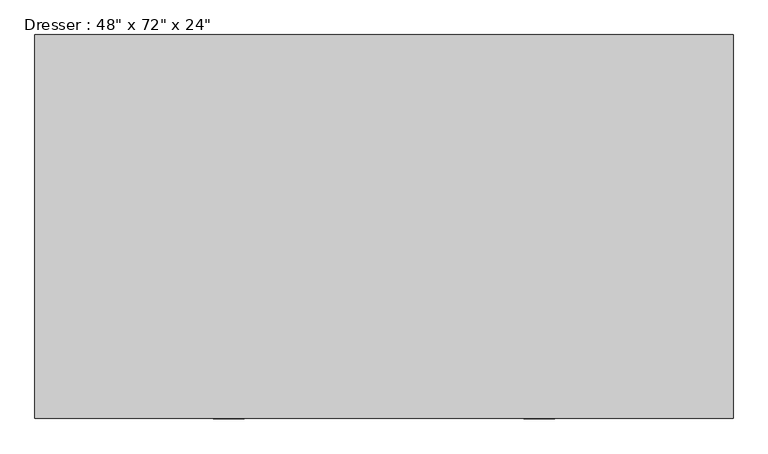
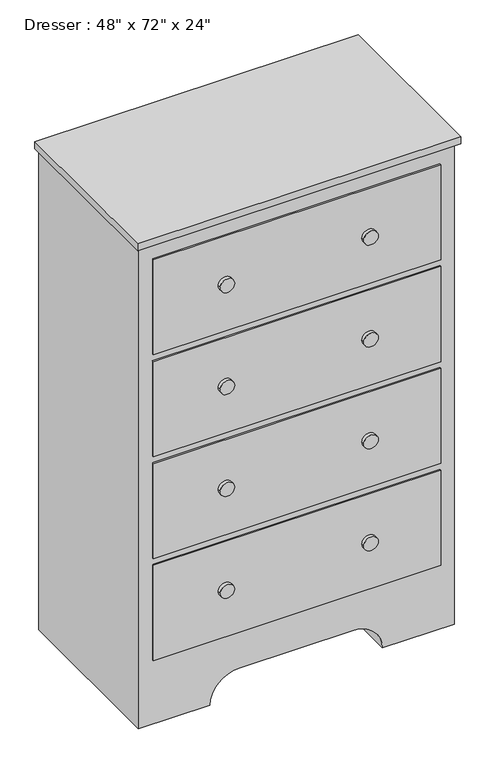
"""IFC4 building model written with IfcOpenShell, lengths in millimetres: furniture geometry."""

from ifc_helpers import new_model, si_unit, point, frame, frame_2d, origin, place, context, project, spatial, polyline, circle_curve, trimmed, segment, composite_curve, outline, extrude, source, transform, mapped, element, save


def furniture_61dbd871(model_context):
    return source(origin(), model_context, "Body", "SweptSolid", [
        extrude(outline(polyline([(302.3067402, -58.3629541), (302.3067402, -687.0129541), (-840.6932598, -687.0129541), (-840.6932598, -58.3629541), (302.3067402, -58.3629541)])), frame((0.0, 0.0, 1803.4), z_axis=(0.0, 0.0, 1.0), x_axis=(1.0, 0.0, 0.0)), (0.0, 0.0, 1.0), 25.4),
        extrude(outline(composite_curve([segment(polyline([(0.0, 289.6067402), (1803.4, 289.6067402), (1803.4, -827.9932598), (0.0, -827.9932598), (0.0, -573.9932598)]), True, "CONTINUOUS"), segment(trimmed(circle_curve(frame_2d((0.0, -472.3932598)), 101.6), [point((0.0, -573.9932598))], [point((101.6, -472.3932598))], True, "CARTESIAN"), True, "CONTINUOUS"), segment(polyline([(101.6, -472.3932598), (101.6, -65.9932598)]), True, "CONTINUOUS"), segment(trimmed(circle_curve(frame_2d((0.0, -65.9932598)), 101.6), [point((101.6, -65.9932598))], [point((0.0, 35.6067402))], True, "CARTESIAN"), True, "CONTINUOUS"), segment(polyline([(0.0, 35.6067402), (0.0, 289.6067402)]), True, "CONTINUOUS")], self_intersect=False)), frame((0.0, -667.9629541, 0.0), z_axis=(0.0, 1.0, 0.0), x_axis=(0.0, 0.0, 1.0)), (0.0, 0.0, 1.0), 609.6),
        extrude(outline(composite_curve([segment(trimmed(circle_curve(frame_2d((1562.1, -15.1932598)), 25.4), [point((1562.1, -40.5932598))], [point((1562.1, 10.2067402))], False, "CARTESIAN"), True, "CONTINUOUS"), segment(trimmed(circle_curve(frame_2d((1562.1, -15.1932598)), 25.4), [point((1562.1, 10.2067402))], [point((1562.1, -40.5932598))], False, "CARTESIAN"), True, "CONTINUOUS")], self_intersect=False)), frame((0.0, -687.0129541, 0.0), z_axis=(0.0, 1.0, 0.0), x_axis=(0.0, 0.0, 1.0)), (0.0, 0.0, 1.0), 12.7),
        extrude(outline(composite_curve([segment(trimmed(circle_curve(frame_2d((1181.1, -15.1932598)), 25.4), [point((1181.1, -40.5932598))], [point((1181.1, 10.2067402))], False, "CARTESIAN"), True, "CONTINUOUS"), segment(trimmed(circle_curve(frame_2d((1181.1, -15.1932598)), 25.4), [point((1181.1, 10.2067402))], [point((1181.1, -40.5932598))], False, "CARTESIAN"), True, "CONTINUOUS")], self_intersect=False)), frame((0.0, -687.0129541, 0.0), z_axis=(0.0, 1.0, 0.0), x_axis=(0.0, 0.0, 1.0)), (0.0, 0.0, 1.0), 12.7),
        extrude(outline(composite_curve([segment(trimmed(circle_curve(frame_2d((800.1, -15.1932598)), 25.4), [point((800.1, -40.5932598))], [point((800.1, 10.2067402))], False, "CARTESIAN"), True, "CONTINUOUS"), segment(trimmed(circle_curve(frame_2d((800.1, -15.1932598)), 25.4), [point((800.1, 10.2067402))], [point((800.1, -40.5932598))], False, "CARTESIAN"), True, "CONTINUOUS")], self_intersect=False)), frame((0.0, -687.0129541, 0.0), z_axis=(0.0, 1.0, 0.0), x_axis=(0.0, 0.0, 1.0)), (0.0, 0.0, 1.0), 12.7),
        extrude(outline(composite_curve([segment(trimmed(circle_curve(frame_2d((419.1, -15.1932598)), 25.4), [point((419.1, -40.5932598))], [point((419.1, 10.2067402))], False, "CARTESIAN"), True, "CONTINUOUS"), segment(trimmed(circle_curve(frame_2d((419.1, -15.1932598)), 25.4), [point((419.1, 10.2067402))], [point((419.1, -40.5932598))], False, "CARTESIAN"), True, "CONTINUOUS")], self_intersect=False)), frame((0.0, -687.0129541, 0.0), z_axis=(0.0, 1.0, 0.0), x_axis=(0.0, 0.0, 1.0)), (0.0, 0.0, 1.0), 12.7),
        extrude(outline(composite_curve([segment(trimmed(circle_curve(frame_2d((419.1, -523.1932598)), 25.4), [point((419.1, -548.5932598))], [point((419.1, -497.7932598))], False, "CARTESIAN"), True, "CONTINUOUS"), segment(trimmed(circle_curve(frame_2d((419.1, -523.1932598)), 25.4), [point((419.1, -497.7932598))], [point((419.1, -548.5932598))], False, "CARTESIAN"), True, "CONTINUOUS")], self_intersect=False)), frame((0.0, -687.0129541, 0.0), z_axis=(0.0, 1.0, 0.0), x_axis=(0.0, 0.0, 1.0)), (0.0, 0.0, 1.0), 12.7),
        extrude(outline(composite_curve([segment(trimmed(circle_curve(frame_2d((800.1, -523.1932598)), 25.4), [point((800.1, -548.5932598))], [point((800.1, -497.7932598))], False, "CARTESIAN"), True, "CONTINUOUS"), segment(trimmed(circle_curve(frame_2d((800.1, -523.1932598)), 25.4), [point((800.1, -497.7932598))], [point((800.1, -548.5932598))], False, "CARTESIAN"), True, "CONTINUOUS")], self_intersect=False)), frame((0.0, -687.0129541, 0.0), z_axis=(0.0, 1.0, 0.0), x_axis=(0.0, 0.0, 1.0)), (0.0, 0.0, 1.0), 12.7),
        extrude(outline(composite_curve([segment(trimmed(circle_curve(frame_2d((1181.1, -523.1932598)), 25.4), [point((1181.1, -548.5932598))], [point((1181.1, -497.7932598))], False, "CARTESIAN"), True, "CONTINUOUS"), segment(trimmed(circle_curve(frame_2d((1181.1, -523.1932598)), 25.4), [point((1181.1, -497.7932598))], [point((1181.1, -548.5932598))], False, "CARTESIAN"), True, "CONTINUOUS")], self_intersect=False)), frame((0.0, -687.0129541, 0.0), z_axis=(0.0, 1.0, 0.0), x_axis=(0.0, 0.0, 1.0)), (0.0, 0.0, 1.0), 12.7),
        extrude(outline(composite_curve([segment(trimmed(circle_curve(frame_2d((1562.1, -523.1932598)), 25.4), [point((1562.1, -548.5932598))], [point((1562.1, -497.7932598))], False, "CARTESIAN"), True, "CONTINUOUS"), segment(trimmed(circle_curve(frame_2d((1562.1, -523.1932598)), 25.4), [point((1562.1, -497.7932598))], [point((1562.1, -548.5932598))], False, "CARTESIAN"), True, "CONTINUOUS")], self_intersect=False)), frame((0.0, -687.0129541, 0.0), z_axis=(0.0, 1.0, 0.0), x_axis=(0.0, 0.0, 1.0)), (0.0, 0.0, 1.0), 12.7),
        extrude(outline(polyline([(238.8067402, -674.3129541), (-777.1932598, -674.3129541), (-777.1932598, -667.9629541), (238.8067402, -667.9629541), (238.8067402, -674.3129541)])), frame((0.0, 0.0, 1384.3), z_axis=(0.0, 0.0, 1.0), x_axis=(1.0, 0.0, 0.0)), (0.0, 0.0, 1.0), 355.6),
        extrude(outline(polyline([(238.8067402, -674.3129541), (-777.1932598, -674.3129541), (-777.1932598, -667.9629541), (238.8067402, -667.9629541), (238.8067402, -674.3129541)])), frame((0.0, 0.0, 1003.3), z_axis=(0.0, 0.0, 1.0), x_axis=(1.0, 0.0, 0.0)), (0.0, 0.0, 1.0), 355.6),
        extrude(outline(polyline([(238.8067402, -674.3129541), (-777.1932598, -674.3129541), (-777.1932598, -667.9629541), (238.8067402, -667.9629541), (238.8067402, -674.3129541)])), frame((0.0, 0.0, 622.3), z_axis=(0.0, 0.0, 1.0), x_axis=(1.0, 0.0, 0.0)), (0.0, 0.0, 1.0), 355.6),
        extrude(outline(polyline([(238.8067402, -674.3129541), (-777.1932598, -674.3129541), (-777.1932598, -667.9629541), (238.8067402, -667.9629541), (238.8067402, -674.3129541)])), frame((0.0, 0.0, 241.3), z_axis=(0.0, 0.0, 1.0), x_axis=(1.0, 0.0, 0.0)), (0.0, 0.0, 1.0), 355.6),
    ])


if __name__ == "__main__":
    model = new_model("IFC4")
    model_context = context("Model", 3, world=origin())
    ifc_project = project(units=[si_unit("LENGTHUNIT", "METRE", prefix="MILLI")], contexts=[model_context])
    site = spatial("IfcSite", under=ifc_project)
    building = spatial("IfcBuilding", under=site)
    placement = place(None, origin())
    furniture_shape = furniture_61dbd871(model_context)
    element("IfcFurniture", 1, ObjectType="Dresser : 48\" x 72\" x 24\"", at=placement, inside=building, context=model_context, shape_type="MappedRepresentation", body=[
        mapped(furniture_shape, transform((0.0, 0.0, 0.0), x_axis=(1.0, 0.0, 0.0), y_axis=(0.0, 1.0, 0.0), z_axis=(0.0, 0.0, 1.0))),
    ])
    save(model, "model.ifc")

# Revit data of these elements
# Type "Dresser : 48\" x 72\" x 24\""
#   Assembly Code = "E2020200"
#   Depth = 2' - 0"
#   Height = 6' - 0"
#   Width = 3' - 8"
#   Dresser Material = Wood Door Panel - Birch
#   Drawer Material = Wood Door Panel - Birch
#   Knob Material = Cherry
#   Default Elevation = 0
# Element 1 (IfcFurniture, "Dresser : 48\" x 72\" x 24\"")
#   Materials on its faces: "Laminate, Ivory, Matte", "Cherry", "Wood Door Panel - Birch"
# Materials
#   "Wood Door Panel - Birch": class "Wood", colour RGB 166 116 52, transparency 0
#   "Cherry": class "Wood", colour RGB 226 177 128, transparency 0, Description = "Prunus Serotina", Cost = 0
#   "Laminate, Ivory, Matte": class "Plastic", colour RGB 247 247 239, transparency 0, Description = "Plastic Laminate - Ivory, Matte", Cost = 0
